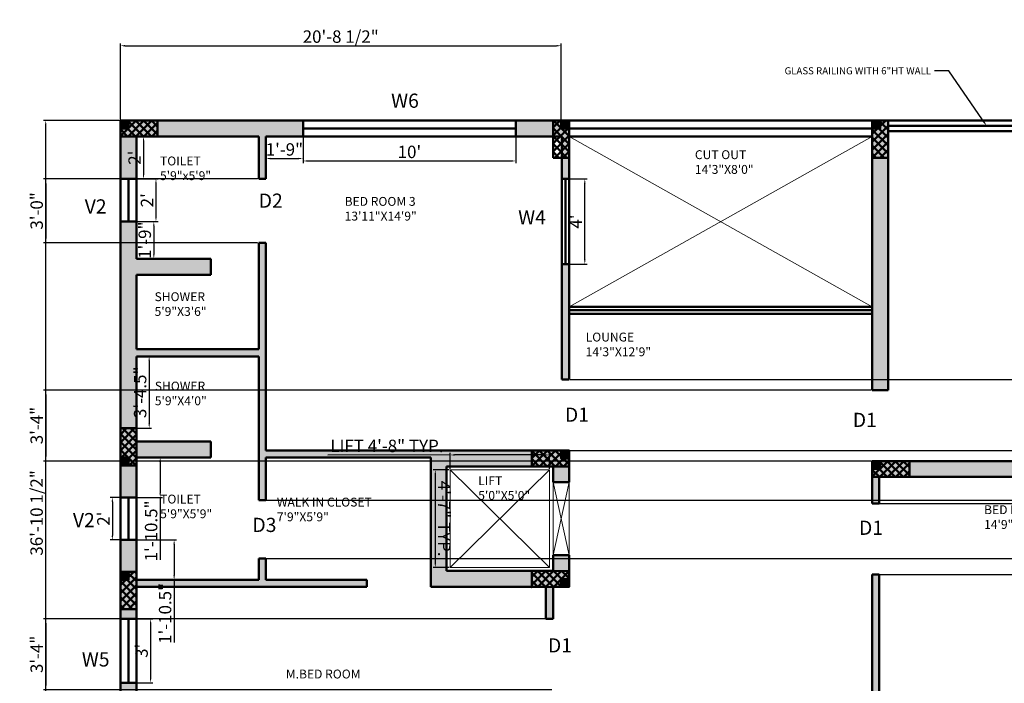
# Model space of a CAD drawing. Units: inches. Extents: x 1749 to 3550, y 1117 to 2383.
# Tile 14 of 15: x 2688 to 3244, y 1992 to 2366. Entities that reach past the tile are written whole.
import ezdxf
from ezdxf import colors
from ezdxf.entities.mleader import LeaderData, LeaderLine
from ezdxf.math import Vec2, Vec3

# ---------------------------------------------------------------- set-up
doc = ezdxf.new("R2010")
doc.units = ezdxf.units.IN
for name, color, linetype, lineweight in [('A-ANNO-DIMS', 2, 'Continuous', 18), ('A-ANNO-SYMB', 1, 'Continuous', 18), ('A-ANNO-TEXT', 3, 'Continuous', 18), ('A-AREA-IDEN', 7, 'Continuous', 18), ('A-COLS', 10, 'Continuous', 50), ('A-EQPM', 8, 'Continuous', 18), ('A-WALL', 7, 'Continuous', 50), ('A-WALL-PATT', 8, 'Continuous', 13)]:
    doc.layers.add(name, color=color, linetype=linetype, lineweight=lineweight)
doc.styles.get("Standard").update_dxf_attribs({"font": 'arial.ttf'})
doc.dimstyles.new('ISO-25', dxfattribs={"dimtxt": 7, "dimasz": 2.5, "dimexe": 1.25, "dimexo": 0.625, "dimtad": 1, "dimdec": 1, "dimlunit": 3, "dimtxsty": 'Standard', "dimcen": 2.5, "dimadec": 0, "dimazin": 0, "dimtfac": 1, "dimtdec": 1, "dimtmove": 0, "dimatfit": 3, "dimfxl": 1, "dimarcsym": 0})

# ---------------------------------------------------------------- blocks, each defined once
blk = doc.blocks.new('*D121')
at = {"layer": 'A-ANNO-DIMS', "color": 0, "lineweight": -2, "ltscale": 0.5, "transparency": 16777216}
for p, q in [((2827.22, 2300.06), (2827.22, 2286.96)), ((2848.22, 2300.06), (2848.22, 2286.96)), ((2829.72, 2288.21), (2845.72, 2288.21))]:
    blk.add_line(p, q, dxfattribs=at)
at = {"layer": 'A-ANNO-DIMS', "color": 0, "ltscale": 0.5, "transparency": 16777216}
for points in [[(2829.72, 2288.62), (2829.72, 2287.79), (2827.22, 2288.21)], [(2845.72, 2288.62), (2845.72, 2287.79), (2848.22, 2288.21)]]:
    blk.add_solid(points, dxfattribs=at)
at = {"layer": 'Defpoints', "color": 0, "ltscale": 0.5, "transparency": 16777216}
for p in [(2827.22, 2300.68), (2848.22, 2300.68), (2848.22, 2288.21)]:
    blk.add_point(p, dxfattribs=at)
at = {"layer": 'A-ANNO-DIMS', "color": 0, "ltscale": 0.5, "transparency": 16777216, "insert": (2837.72, 2292.41), "char_height": 7, "attachment_point": 5}
blk.add_mtext('1\'-9"', dxfattribs=at)
blk = doc.blocks.new('*D122')
at = {"layer": 'A-ANNO-DIMS', "color": 0, "lineweight": -2, "ltscale": 0.5, "transparency": 16777216}
for p, q in [((2848.22, 2300.06), (2848.22, 2285.58)), ((2968.22, 2300.06), (2968.22, 2285.58)), ((2850.72, 2286.83), (2965.72, 2286.83))]:
    blk.add_line(p, q, dxfattribs=at)
at = {"layer": 'A-ANNO-DIMS', "color": 0, "ltscale": 0.5, "transparency": 16777216}
for points in [[(2850.72, 2287.24), (2850.72, 2286.41), (2848.22, 2286.83)], [(2965.72, 2287.24), (2965.72, 2286.41), (2968.22, 2286.83)]]:
    blk.add_solid(points, dxfattribs=at)
at = {"layer": 'Defpoints', "color": 0, "ltscale": 0.5, "transparency": 16777216}
for p in [(2848.22, 2300.68), (2968.22, 2300.68), (2968.22, 2286.83)]:
    blk.add_point(p, dxfattribs=at)
at = {"layer": 'A-ANNO-DIMS', "color": 0, "ltscale": 0.5, "transparency": 16777216, "insert": (2908.22, 2291.03), "char_height": 7, "attachment_point": 5}
blk.add_mtext("10'", dxfattribs=at)
blk = doc.blocks.new('*D123')
at = {"layer": 'A-ANNO-DIMS', "color": 0, "lineweight": -2, "ltscale": 0.5, "transparency": 16777216}
for p, q in [((2754.84, 2300.68), (2759.52, 2300.68)), ((2758.27, 2298.18), (2758.27, 2279.18)), ((2754.84, 2276.68), (2759.52, 2276.68))]:
    blk.add_line(p, q, dxfattribs=at)
at = {"layer": 'A-ANNO-DIMS', "color": 0, "ltscale": 0.5, "transparency": 16777216}
for points in [[(2757.85, 2298.18), (2758.68, 2298.18), (2758.27, 2300.68)], [(2757.85, 2279.18), (2758.68, 2279.18), (2758.27, 2276.68)]]:
    blk.add_solid(points, dxfattribs=at)
at = {"layer": 'Defpoints', "color": 0, "ltscale": 0.5, "transparency": 16777216}
for p in [(2754.22, 2300.68), (2754.22, 2276.68), (2758.27, 2276.68)]:
    blk.add_point(p, dxfattribs=at)
at = {"layer": 'A-ANNO-DIMS', "color": 0, "ltscale": 0.5, "transparency": 16777216, "insert": (2754.13, 2288.68), "char_height": 7, "attachment_point": 5, "rotation": 90}
blk.add_mtext("2'", dxfattribs=at)
blk = doc.blocks.new('*D124')
at = {"layer": 'A-ANNO-DIMS', "color": 0, "lineweight": -2, "ltscale": 0.5, "transparency": 16777216}
for p, q in [((2754.84, 2276.68), (2766.53, 2276.68)), ((2765.28, 2274.18), (2765.28, 2255.18)), ((2754.84, 2252.68), (2766.53, 2252.68))]:
    blk.add_line(p, q, dxfattribs=at)
at = {"layer": 'A-ANNO-DIMS', "color": 0, "ltscale": 0.5, "transparency": 16777216}
for points in [[(2764.86, 2274.18), (2765.69, 2274.18), (2765.28, 2276.68)], [(2764.86, 2255.18), (2765.69, 2255.18), (2765.28, 2252.68)]]:
    blk.add_solid(points, dxfattribs=at)
at = {"layer": 'Defpoints', "color": 0, "ltscale": 0.5, "transparency": 16777216}
for p in [(2754.22, 2276.68), (2754.22, 2252.68), (2765.28, 2252.68)]:
    blk.add_point(p, dxfattribs=at)
at = {"layer": 'A-ANNO-DIMS', "color": 0, "ltscale": 0.5, "transparency": 16777216, "insert": (2761.14, 2264.68), "char_height": 7, "attachment_point": 5, "rotation": 90}
blk.add_mtext("2'", dxfattribs=at)
blk = doc.blocks.new('*D125')
at = {"layer": 'A-ANNO-DIMS', "color": 0, "lineweight": -2, "ltscale": 0.5, "transparency": 16777216}
for p, q in [((2754.84, 2252.68), (2765.33, 2252.68)), ((2764.08, 2250.18), (2764.08, 2234.18)), ((2754.84, 2231.68), (2765.33, 2231.68))]:
    blk.add_line(p, q, dxfattribs=at)
at = {"layer": 'A-ANNO-DIMS', "color": 0, "ltscale": 0.5, "transparency": 16777216}
for points in [[(2763.66, 2250.18), (2764.49, 2250.18), (2764.08, 2252.68)], [(2763.66, 2234.18), (2764.49, 2234.18), (2764.08, 2231.68)]]:
    blk.add_solid(points, dxfattribs=at)
at = {"layer": 'Defpoints', "color": 0, "ltscale": 0.5, "transparency": 16777216}
for p in [(2754.22, 2252.68), (2754.22, 2231.68), (2764.08, 2231.68)]:
    blk.add_point(p, dxfattribs=at)
at = {"layer": 'A-ANNO-DIMS', "color": 0, "ltscale": 0.5, "transparency": 16777216, "insert": (2759.88, 2242.18), "char_height": 7, "attachment_point": 5, "rotation": 90}
blk.add_mtext('1\'-9"', dxfattribs=at)
blk = doc.blocks.new('*D126')
at = {"layer": 'A-ANNO-DIMS', "color": 0, "lineweight": -2, "ltscale": 0.5, "transparency": 16777216}
for p, q in [((2754.84, 2176.68), (2762.7, 2176.68)), ((2761.45, 2174.18), (2761.45, 2138.68)), ((2754.84, 2136.18), (2762.7, 2136.18))]:
    blk.add_line(p, q, dxfattribs=at)
at = {"layer": 'A-ANNO-DIMS', "color": 0, "ltscale": 0.5, "transparency": 16777216}
for points in [[(2761.03, 2174.18), (2761.87, 2174.18), (2761.45, 2176.68)], [(2761.03, 2138.68), (2761.87, 2138.68), (2761.45, 2136.18)]]:
    blk.add_solid(points, dxfattribs=at)
at = {"layer": 'Defpoints', "color": 0, "ltscale": 0.5, "transparency": 16777216}
for p in [(2754.22, 2176.68), (2754.22, 2136.18), (2761.45, 2136.18)]:
    blk.add_point(p, dxfattribs=at)
at = {"layer": 'A-ANNO-DIMS', "color": 0, "ltscale": 0.5, "transparency": 16777216, "insert": (2757.25, 2156.43), "char_height": 7, "attachment_point": 5, "rotation": 90}
blk.add_mtext('3\'-4.5"', dxfattribs=at)
blk = doc.blocks.new('*D127')
at = {"layer": 'A-ANNO-DIMS', "color": 0, "lineweight": -2, "ltscale": 0.5, "transparency": 16777216}
for p, q in [((2754.84, 2119.68), (2768.9, 2119.68)), ((2767.65, 2117.18), (2767.65, 2099.68)), ((2754.84, 2097.18), (2768.9, 2097.18)), ((2767.65, 2097.18), (2767.65, 2061.89))]:
    blk.add_line(p, q, dxfattribs=at)
at = {"layer": 'A-ANNO-DIMS', "color": 0, "ltscale": 0.5, "transparency": 16777216}
for points in [[(2767.24, 2117.18), (2768.07, 2117.18), (2767.65, 2119.68)], [(2767.24, 2099.68), (2768.07, 2099.68), (2767.65, 2097.18)]]:
    blk.add_solid(points, dxfattribs=at)
at = {"layer": 'Defpoints', "color": 0, "ltscale": 0.5, "transparency": 16777216}
for p in [(2754.22, 2119.68), (2754.22, 2097.18), (2767.65, 2097.18)]:
    blk.add_point(p, dxfattribs=at)
at = {"layer": 'A-ANNO-DIMS', "color": 0, "ltscale": 0.5, "transparency": 16777216, "insert": (2763.45, 2078.28), "char_height": 7, "attachment_point": 5, "rotation": 90}
blk.add_mtext('1\'-10.5"', dxfattribs=at)
blk = doc.blocks.new('*D128')
at = {"layer": 'A-ANNO-DIMS', "color": 0, "lineweight": -2, "ltscale": 0.5, "transparency": 16777216}
for p, q in [((2744.59, 2097.18), (2739.43, 2097.18)), ((2740.68, 2094.68), (2740.68, 2075.68)), ((2744.59, 2073.18), (2739.43, 2073.18))]:
    blk.add_line(p, q, dxfattribs=at)
at = {"layer": 'A-ANNO-DIMS', "color": 0, "ltscale": 0.5, "transparency": 16777216}
for points in [[(2740.26, 2094.68), (2741.09, 2094.68), (2740.68, 2097.18)], [(2740.26, 2075.68), (2741.09, 2075.68), (2740.68, 2073.18)]]:
    blk.add_solid(points, dxfattribs=at)
at = {"layer": 'Defpoints', "color": 0, "ltscale": 0.5, "transparency": 16777216}
for p in [(2745.22, 2097.18), (2740.68, 2073.18), (2745.22, 2073.18)]:
    blk.add_point(p, dxfattribs=at)
at = {"layer": 'A-ANNO-DIMS', "color": 0, "ltscale": 0.5, "transparency": 16777216, "insert": (2736.54, 2085.18), "char_height": 7, "attachment_point": 5, "rotation": 90}
blk.add_mtext("2'", dxfattribs=at)
blk = doc.blocks.new('*D129')
at = {"layer": 'A-ANNO-DIMS', "color": 0, "lineweight": -2, "ltscale": 0.5, "transparency": 16777216}
for p, q in [((2754.84, 2073.18), (2776.78, 2073.18)), ((2775.53, 2070.68), (2775.53, 2053.18)), ((2754.84, 2050.68), (2776.78, 2050.68)), ((2775.53, 2050.68), (2775.53, 2015.39))]:
    blk.add_line(p, q, dxfattribs=at)
at = {"layer": 'A-ANNO-DIMS', "color": 0, "ltscale": 0.5, "transparency": 16777216}
for points in [[(2775.11, 2070.68), (2775.94, 2070.68), (2775.53, 2073.18)], [(2775.11, 2053.18), (2775.94, 2053.18), (2775.53, 2050.68)]]:
    blk.add_solid(points, dxfattribs=at)
at = {"layer": 'Defpoints', "color": 0, "ltscale": 0.5, "transparency": 16777216}
for p in [(2754.22, 2073.18), (2754.22, 2050.68), (2775.53, 2050.68)]:
    blk.add_point(p, dxfattribs=at)
at = {"layer": 'A-ANNO-DIMS', "color": 0, "ltscale": 0.5, "transparency": 16777216, "insert": (2771.33, 2031.78), "char_height": 7, "attachment_point": 5, "rotation": 90}
blk.add_mtext('1\'-10.5"', dxfattribs=at)
blk = doc.blocks.new('*D130')
at = {"layer": 'A-ANNO-DIMS', "color": 0, "lineweight": -2, "ltscale": 0.5, "transparency": 16777216}
for p, q in [((2754.84, 2028.68), (2763.51, 2028.68)), ((2762.26, 2026.18), (2762.26, 1995.18)), ((2754.84, 1992.68), (2763.51, 1992.68))]:
    blk.add_line(p, q, dxfattribs=at)
at = {"layer": 'A-ANNO-DIMS', "color": 0, "ltscale": 0.5, "transparency": 16777216}
for points in [[(2761.85, 2026.18), (2762.68, 2026.18), (2762.26, 2028.68)], [(2761.85, 1995.18), (2762.68, 1995.18), (2762.26, 1992.68)]]:
    blk.add_solid(points, dxfattribs=at)
at = {"layer": 'Defpoints', "color": 0, "ltscale": 0.5, "transparency": 16777216}
for p in [(2754.22, 2028.68), (2754.22, 1992.68), (2762.26, 1992.68)]:
    blk.add_point(p, dxfattribs=at)
at = {"layer": 'A-ANNO-DIMS', "color": 0, "ltscale": 0.5, "transparency": 16777216, "insert": (2758.06, 2010.68), "char_height": 7, "attachment_point": 5, "rotation": 90}
blk.add_mtext("3'", dxfattribs=at)
blk = doc.blocks.new('*D137')
at = {"layer": 'A-ANNO-DIMS', "color": 0, "lineweight": -2, "ltscale": 0.5, "transparency": 16777216}
for p, q in [((2998.84, 2276.68), (3008.38, 2276.68)), ((3007.13, 2231.18), (3007.13, 2274.18)), ((2998.84, 2228.68), (3008.38, 2228.68))]:
    blk.add_line(p, q, dxfattribs=at)
at = {"layer": 'A-ANNO-DIMS', "color": 0, "ltscale": 0.5, "transparency": 16777216}
for points in [[(3006.71, 2274.18), (3007.55, 2274.18), (3007.13, 2276.68)], [(3006.71, 2231.18), (3007.55, 2231.18), (3007.13, 2228.68)]]:
    blk.add_solid(points, dxfattribs=at)
at = {"layer": 'Defpoints', "color": 0, "ltscale": 0.5, "transparency": 16777216}
for p in [(2998.22, 2276.68), (3007.13, 2276.68), (2998.22, 2228.68)]:
    blk.add_point(p, dxfattribs=at)
at = {"layer": 'A-ANNO-DIMS', "color": 0, "ltscale": 0.5, "transparency": 16777216, "insert": (3003, 2252.68), "char_height": 7, "attachment_point": 5, "rotation": 90}
blk.add_mtext("4'", dxfattribs=at)
blk = doc.blocks.new('LIFT-B')
at = {"ltscale": 0.5}
for p, q in [((0, 55), (56, 55)), ((0, 0), (0, 55)), ((56, 55), (0, 0)), ((0, 55), (56, 0)), ((56, 55), (56, 0)), ((56, 0), (0, 0))]:
    blk.add_line(p, q, dxfattribs=at)
blk = doc.blocks.new('*D155')
at = {"layer": 'A-ANNO-DIMS', "color": 0, "lineweight": -2, "ltscale": 0.5, "transparency": 16777216}
for p, q in [((2931.22, 2113.31), (2931.22, 2122.33)), ((2987.22, 2113.31), (2987.22, 2122.33)), ((2931.22, 2121.08), (2862.29, 2121.07)), ((2984.72, 2121.08), (2933.72, 2121.08))]:
    blk.add_line(p, q, dxfattribs=at)
at = {"layer": 'A-ANNO-DIMS', "color": 0, "ltscale": 0.5, "transparency": 16777216}
for points in [[(2933.72, 2121.5), (2933.72, 2120.66), (2931.22, 2121.08)], [(2984.72, 2121.5), (2984.72, 2120.67), (2987.22, 2121.08)]]:
    blk.add_solid(points, dxfattribs=at)
at = {"layer": 'Defpoints', "color": 0, "ltscale": 0.5, "transparency": 16777216}
for p in [(2931.22, 2121.08), (2931.22, 2112.68), (2987.22, 2112.68)]:
    blk.add_point(p, dxfattribs=at)
at = {"layer": 'A-ANNO-DIMS', "color": 0, "ltscale": 0.5, "transparency": 16777216, "insert": (2895.51, 2125.28), "char_height": 7, "attachment_point": 5, "rotation": 0.0046}
blk.add_mtext('LIFT 4\'-8" TYP.', dxfattribs=at)
blk = doc.blocks.new('*D156')
at = {"layer": 'A-ANNO-DIMS', "color": 0, "lineweight": -2, "ltscale": 0.5, "transparency": 16777216}
for p, q in [((2930.6, 2112.68), (2921.57, 2112.68)), ((2922.82, 2110.18), (2922.83, 2060.18)), ((2930.6, 2057.68), (2921.58, 2057.68))]:
    blk.add_line(p, q, dxfattribs=at)
at = {"layer": 'A-ANNO-DIMS', "color": 0, "ltscale": 0.5, "transparency": 16777216}
for points in [[(2923.24, 2110.18), (2922.41, 2110.18), (2922.82, 2112.68)], [(2923.24, 2060.18), (2922.41, 2060.18), (2922.83, 2057.68)]]:
    blk.add_solid(points, dxfattribs=at)
at = {"layer": 'Defpoints', "color": 0, "ltscale": 0.5, "transparency": 16777216}
for p in [(2931.22, 2112.68), (2922.83, 2057.68), (2931.23, 2057.68)]:
    blk.add_point(p, dxfattribs=at)
at = {"layer": 'A-ANNO-DIMS', "color": 0, "ltscale": 0.5, "transparency": 16777216, "insert": (2926.95, 2085.18), "char_height": 7, "attachment_point": 5, "rotation": 270.0046}
blk.add_mtext('4\'-7" TYP.', dxfattribs=at)
blk = doc.blocks.new('*D181')
at = {"layer": 'A-ANNO-DIMS', "color": 0, "lineweight": -2, "ltscale": 0.5, "transparency": 16777216}
for p, q in [((2744.59, 2309.68), (2701.86, 2309.68)), ((2703.11, 1869.68), (2703.11, 2307.18)), ((2744.59, 1867.18), (2701.86, 1867.18))]:
    blk.add_line(p, q, dxfattribs=at)
at = {"layer": 'A-ANNO-DIMS', "color": 0, "ltscale": 0.5, "transparency": 16777216}
for points in [[(2702.69, 2307.18), (2703.52, 2307.18), (2703.11, 2309.68)], [(2702.69, 1869.68), (2703.52, 1869.68), (2703.11, 1867.18)]]:
    blk.add_solid(points, dxfattribs=at)
at = {"layer": 'Defpoints', "color": 0, "ltscale": 0.5, "transparency": 16777216}
for p in [(2703.11, 2309.68), (2745.22, 2309.68), (2745.22, 1867.18)]:
    blk.add_point(p, dxfattribs=at)
at = {"layer": 'A-ANNO-DIMS', "color": 0, "ltscale": 0.5, "transparency": 16777216, "insert": (2698.86, 2088.43), "char_height": 7, "attachment_point": 5, "rotation": 90}
blk.add_mtext('36\'-10 1/2"', dxfattribs=at)
blk = doc.blocks.new('*D182')
at = {"layer": 'A-ANNO-DIMS', "color": 0, "lineweight": -2, "ltscale": 0.5, "transparency": 16777216}
for p, q in [((2745.22, 2310.31), (2745.22, 2353.03)), ((2747.72, 2351.78), (2991.22, 2351.78)), ((2993.72, 2310.31), (2993.72, 2353.03))]:
    blk.add_line(p, q, dxfattribs=at)
at = {"layer": 'A-ANNO-DIMS', "color": 0, "ltscale": 0.5, "transparency": 16777216}
for points in [[(2747.72, 2352.2), (2747.72, 2351.36), (2745.22, 2351.78)], [(2991.22, 2352.2), (2991.22, 2351.36), (2993.72, 2351.78)]]:
    blk.add_solid(points, dxfattribs=at)
at = {"layer": 'Defpoints', "color": 0, "ltscale": 0.5, "transparency": 16777216}
for p in [(2993.72, 2351.78), (2745.22, 2309.68), (2993.72, 2309.68)]:
    blk.add_point(p, dxfattribs=at)
at = {"layer": 'A-ANNO-DIMS', "color": 0, "ltscale": 0.5, "transparency": 16777216, "insert": (2869.47, 2356.03), "char_height": 7, "attachment_point": 5}
blk.add_mtext('20\'-8 1/2"', dxfattribs=at)
blk = doc.blocks.new('*D191')
at = {"layer": 'A-ANNO-DIMS', "color": 0, "lineweight": -2, "ltscale": 0.5, "transparency": 16777216}
for p, q in [((2998.84, 2163.68), (3455.57, 2163.68)), ((3454.32, 2161.18), (3454.32, 2126.18)), ((2998.84, 2123.68), (3455.57, 2123.68))]:
    blk.add_line(p, q, dxfattribs=at)
at = {"layer": 'A-ANNO-DIMS', "color": 0, "ltscale": 0.5, "transparency": 16777216}
for points in [[(3453.9, 2161.18), (3454.74, 2161.18), (3454.32, 2163.68)], [(3453.9, 2126.18), (3454.74, 2126.18), (3454.32, 2123.68)]]:
    blk.add_solid(points, dxfattribs=at)
at = {"layer": 'Defpoints', "color": 0, "ltscale": 0.5, "transparency": 16777216}
for p in [(2998.22, 2163.68), (2998.22, 2123.68), (3454.32, 2123.68)]:
    blk.add_point(p, dxfattribs=at)
at = {"layer": 'A-ANNO-DIMS', "color": 0, "ltscale": 0.5, "transparency": 16777216, "insert": (3450.12, 2143.68), "char_height": 7, "attachment_point": 5, "rotation": 90}
blk.add_mtext('3\'-4"', dxfattribs=at)
blk = doc.blocks.new('*D192')
at = {"layer": 'A-ANNO-DIMS', "color": 0, "lineweight": -2, "ltscale": 0.5, "transparency": 16777216}
for p, q in [((3168.59, 2157.68), (2701.86, 2157.68)), ((2703.11, 2155.18), (2703.11, 2120.18)), ((3168.59, 2117.68), (2701.86, 2117.68))]:
    blk.add_line(p, q, dxfattribs=at)
at = {"layer": 'A-ANNO-DIMS', "color": 0, "ltscale": 0.5, "transparency": 16777216}
for points in [[(2702.69, 2155.18), (2703.52, 2155.18), (2703.11, 2157.68)], [(2702.69, 2120.18), (2703.52, 2120.18), (2703.11, 2117.68)]]:
    blk.add_solid(points, dxfattribs=at)
at = {"layer": 'Defpoints', "color": 0, "ltscale": 0.5, "transparency": 16777216}
for p in [(3169.22, 2157.68), (2703.11, 2117.68), (3169.22, 2117.68)]:
    blk.add_point(p, dxfattribs=at)
at = {"layer": 'A-ANNO-DIMS', "color": 0, "ltscale": 0.5, "transparency": 16777216, "insert": (2698.91, 2137.68), "char_height": 7, "attachment_point": 5, "rotation": 90}
blk.add_mtext('3\'-4"', dxfattribs=at)
blk = doc.blocks.new('*D193')
at = {"layer": 'A-ANNO-DIMS', "color": 0, "lineweight": -2, "ltscale": 0.5, "transparency": 16777216}
for p, q in [((3169.84, 2093.68), (3455.57, 2093.68)), ((3454.32, 2091.18), (3454.32, 2056.18)), ((3169.84, 2053.68), (3455.57, 2053.68))]:
    blk.add_line(p, q, dxfattribs=at)
at = {"layer": 'A-ANNO-DIMS', "color": 0, "ltscale": 0.5, "transparency": 16777216}
for points in [[(3453.9, 2091.18), (3454.74, 2091.18), (3454.32, 2093.68)], [(3453.9, 2056.18), (3454.74, 2056.18), (3454.32, 2053.68)]]:
    blk.add_solid(points, dxfattribs=at)
at = {"layer": 'Defpoints', "color": 0, "ltscale": 0.5, "transparency": 16777216}
for p in [(3169.22, 2093.68), (3169.22, 2053.68), (3454.32, 2053.68)]:
    blk.add_point(p, dxfattribs=at)
at = {"layer": 'A-ANNO-DIMS', "color": 0, "ltscale": 0.5, "transparency": 16777216, "insert": (3450.12, 2073.68), "char_height": 7, "attachment_point": 5, "rotation": 90}
blk.add_mtext('3\'-4"', dxfattribs=at)
blk = doc.blocks.new('*D194')
at = {"layer": 'A-ANNO-DIMS', "color": 0, "lineweight": -2, "ltscale": 0.5, "transparency": 16777216}
for p, q in [((2988.59, 2028.68), (2701.86, 2028.68)), ((2703.11, 2026.18), (2703.11, 1991.18)), ((2988.59, 1988.68), (2701.86, 1988.68))]:
    blk.add_line(p, q, dxfattribs=at)
at = {"layer": 'A-ANNO-DIMS', "color": 0, "ltscale": 0.5, "transparency": 16777216}
for points in [[(2702.69, 2026.18), (2703.52, 2026.18), (2703.11, 2028.68)], [(2702.69, 1991.18), (2703.52, 1991.18), (2703.11, 1988.68)]]:
    blk.add_solid(points, dxfattribs=at)
at = {"layer": 'Defpoints', "color": 0, "ltscale": 0.5, "transparency": 16777216}
for p in [(2989.22, 2028.68), (2703.11, 1988.68), (2989.22, 1988.68)]:
    blk.add_point(p, dxfattribs=at)
at = {"layer": 'A-ANNO-DIMS', "color": 0, "ltscale": 0.5, "transparency": 16777216, "insert": (2698.91, 2008.68), "char_height": 7, "attachment_point": 5, "rotation": 90}
blk.add_mtext('3\'-4"', dxfattribs=at)
blk = doc.blocks.new('*D195')
at = {"layer": 'A-ANNO-DIMS', "color": 0, "lineweight": -2, "ltscale": 0.5, "transparency": 16777216}
for p, q in [((2822.59, 2276.68), (2701.86, 2276.68)), ((2703.11, 2274.18), (2703.11, 2243.18)), ((2822.59, 2240.68), (2701.86, 2240.68))]:
    blk.add_line(p, q, dxfattribs=at)
at = {"layer": 'A-ANNO-DIMS', "color": 0, "ltscale": 0.5, "transparency": 16777216}
for points in [[(2702.69, 2274.18), (2703.52, 2274.18), (2703.11, 2276.68)], [(2702.69, 2243.18), (2703.52, 2243.18), (2703.11, 2240.68)]]:
    blk.add_solid(points, dxfattribs=at)
at = {"layer": 'Defpoints', "color": 0, "ltscale": 0.5, "transparency": 16777216}
for p in [(2823.22, 2276.68), (2703.11, 2240.68), (2823.22, 2240.68)]:
    blk.add_point(p, dxfattribs=at)
at = {"layer": 'A-ANNO-DIMS', "color": 0, "ltscale": 0.5, "transparency": 16777216, "insert": (2698.91, 2258.68), "char_height": 7, "attachment_point": 5, "rotation": 90}
blk.add_mtext('3\'-0"', dxfattribs=at)
blk = doc.blocks.new('*D197')
at = {"layer": 'A-ANNO-DIMS', "color": 0, "lineweight": -2, "ltscale": 0.5, "transparency": 16777216}
for p, q in [((2823.84, 2095.68), (3455.57, 2095.68)), ((3454.32, 2093.18), (3454.32, 2065.18)), ((2823.84, 2062.68), (3455.57, 2062.68))]:
    blk.add_line(p, q, dxfattribs=at)
at = {"layer": 'A-ANNO-DIMS', "color": 0, "ltscale": 0.5, "transparency": 16777216}
for points in [[(3453.9, 2093.18), (3454.74, 2093.18), (3454.32, 2095.68)], [(3453.9, 2065.18), (3454.74, 2065.18), (3454.32, 2062.68)]]:
    blk.add_solid(points, dxfattribs=at)
at = {"layer": 'Defpoints', "color": 0, "ltscale": 0.5, "transparency": 16777216}
for p in [(2823.22, 2095.68), (2823.22, 2062.68), (3454.32, 2062.68)]:
    blk.add_point(p, dxfattribs=at)
at = {"layer": 'A-ANNO-DIMS', "color": 0, "ltscale": 0.5, "transparency": 16777216, "insert": (3450.12, 2079.18), "char_height": 7, "attachment_point": 5, "rotation": 90}
blk.add_mtext('2\'-9"', dxfattribs=at)

msp = doc.modelspace()

# ---------------------------------------------------------------- hatches: boundary and pattern name
at = {"layer": 'A-COLS', "ltscale": 10}
h = msp.add_hatch(color=256, dxfattribs=at)
h.dxf.hatch_style = 1
h.paths.add_polyline_path([(2745.22, 2305.18), (2749.72, 2305.18), (2749.72, 2309.68), (2745.22, 2309.68)])
h = msp.add_hatch(dxfattribs=at)
h.set_pattern_fill('ANSI37', color=256, angle=180)
h.set_pattern_definition([(225, (4417.464, 3667.787), (2.245064, -2.245064), []), (315, (4417.464, 3667.787), (2.245064, 2.245064), [])])
h.paths.add_polyline_path([(2745.22, 2309.68), (2745.22, 2300.68), (2766.22, 2300.68), (2766.22, 2309.68)])
h = msp.add_hatch(dxfattribs=at)
h.set_pattern_fill('ANSI37', color=256, angle=90)
h.set_pattern_definition([(135, (4356.3257, 637.4367), (-2.245064, -2.245064), []), (225, (4356.3257, 637.4367), (2.245064, -2.245064), [])])
h.paths.add_polyline_path([(2998.22, 2309.68), (2989.22, 2309.68), (2989.22, 2288.68), (2998.22, 2288.68)])
h = msp.add_hatch(color=256, dxfattribs=at)
h.dxf.hatch_style = 1
h.paths.add_polyline_path([(2993.72, 2309.68), (2993.72, 2305.18), (2998.22, 2305.18), (2998.22, 2309.68)])
h = msp.add_hatch(color=256, dxfattribs=at)
h.dxf.hatch_style = 1
h.paths.add_polyline_path([(3169.22, 2309.68), (3169.22, 2305.18), (3173.72, 2305.18), (3173.72, 2309.68)])
h = msp.add_hatch(dxfattribs=at)
h.set_pattern_fill('ANSI37', color=256, angle=90)
h.set_pattern_definition([(135, (4508.4704, 637.4367), (-2.245064, -2.245064), []), (225, (4508.4704, 637.4367), (2.245064, -2.245064), [])])
h.paths.add_polyline_path([(3169.22, 2288.68), (3178.22, 2288.68), (3178.22, 2309.68), (3169.22, 2309.68)])
h = msp.add_hatch(dxfattribs=at)
h.set_pattern_fill('ANSI37', color=256, angle=270)
h.set_pattern_definition([(315, (1387.1012, 3787.4255), (2.245064, 2.245064), []), (45, (1387.1012, 3787.4255), (-2.245064, 2.245064), [])])
h.paths.add_polyline_path([(2745.21, 2115.18), (2754.21, 2115.18), (2754.21, 2136.18), (2745.21, 2136.18)])
h = msp.add_hatch(dxfattribs=at)
h.set_pattern_fill('ANSI37', color=256, angle=180)
h.set_pattern_definition([(225, (4694.5, 3481.787), (2.245064, -2.245064), []), (315, (4694.5, 3481.787), (2.245064, 2.245064), [])])
h.paths.add_polyline_path([(2977.22, 2123.68), (2977.22, 2114.68), (2998.22, 2114.68), (2998.22, 2123.68)])
h = msp.add_hatch(color=256, dxfattribs=at)
h.dxf.hatch_style = 1
h.paths.add_polyline_path([(2998.22, 2123.68), (2993.72, 2123.68), (2993.72, 2119.18), (2998.22, 2119.18)])
h = msp.add_hatch(color=256, dxfattribs=at)
h.dxf.hatch_style = 1
h.paths.add_polyline_path([(2749.71, 2115.18), (2749.71, 2119.68), (2745.21, 2119.68), (2745.21, 2115.18)])
h = msp.add_hatch(color=256, dxfattribs=at)
h.dxf.hatch_style = 1
h.paths.add_polyline_path([(3169.22, 2113.18), (3173.72, 2113.18), (3173.72, 2117.68), (3169.22, 2117.68)])
h = msp.add_hatch(dxfattribs=at)
h.set_pattern_fill('ANSI37', color=256, angle=180)
h.set_pattern_definition([(225, (4841.464, 3475.787), (2.245064, -2.245064), []), (315, (4841.464, 3475.787), (2.245064, 2.245064), [])])
h.paths.add_polyline_path([(3169.22, 2117.68), (3169.22, 2108.68), (3190.22, 2108.68), (3190.22, 2117.68)])
h = msp.add_hatch(color=256, dxfattribs=at)
h.dxf.hatch_style = 1
h.paths.add_polyline_path([(2745.22, 2055.15), (2745.22, 2050.65), (2749.72, 2050.65), (2749.72, 2055.15)])
h = msp.add_hatch(dxfattribs=at)
h.set_pattern_fill('ANSI37', color=256, angle=90)
h.set_pattern_definition([(135, (4079.926, 382.902), (-2.245064, -2.245064), []), (225, (4079.926, 382.902), (2.245064, -2.245064), [])])
h.paths.add_polyline_path([(2745.22, 2034.15), (2754.22, 2034.15), (2754.22, 2055.15), (2745.22, 2055.15)])
h = msp.add_hatch(dxfattribs=at)
h.set_pattern_fill('ANSI37', color=256, angle=0.3283)
h.set_pattern_definition([(45.32827, (1333.7838, 679.0164), (-2.25789, 2.2321643), []), (135.32827, (1333.7838, 679.0164), (-2.2321643, -2.25789), [])])
h.paths.add_polyline_path([(2998.22, 2046.68), (2998.17, 2055.68), (2977.17, 2055.56), (2977.22, 2046.56)])
h = msp.add_hatch(color=256, dxfattribs=at)
h.dxf.hatch_style = 1
h.paths.add_polyline_path([(2998.19, 2051.18), (2993.69, 2051.16), (2993.72, 2046.66), (2998.22, 2046.68)])
at = {"layer": 'A-WALL-PATT', "ltscale": 0.5}
h = msp.add_hatch(color=256, dxfattribs=at)
h.dxf.hatch_style = 1
h.paths.add_polyline_path([(2745.22, 2309.68), (2745.22, 2276.68), (2754.22, 2276.68), (2754.22, 2300.68), (2823.22, 2300.68), (2823.22, 2276.68), (2827.22, 2276.68), (2827.22, 2300.68), (2848.22, 2300.68), (2848.22, 2309.68)])
h = msp.add_hatch(color=256, dxfattribs=at)
h.dxf.hatch_style = 1
h.paths.add_polyline_path([(2968.22, 2309.68), (2968.22, 2300.68), (2994.22, 2300.68), (2994.22, 2276.68), (2998.22, 2276.68), (2998.22, 2300.68), (2998.22, 2309.68)])
h = msp.add_hatch(color=256, dxfattribs=at)
h.dxf.hatch_style = 1
h.paths.add_polyline_path([(3169.22, 2157.68), (3178.22, 2157.68), (3178.22, 2303.68), (3178.22, 2309.68), (3169.22, 2309.68), (3169.22, 2300.68), (3169.22, 2204.68), (3169.22, 2200.68)])
h = msp.add_hatch(color=256, dxfattribs=at)
h.dxf.hatch_style = 1
h.paths.add_polyline_path([(2929.22, 2055.68), (2929.22, 2114.68), (2989.22, 2114.68), (2989.22, 2105.68), (2998.22, 2105.68), (2998.22, 2123.68), (2827.22, 2123.68), (2827.22, 2240.68), (2823.22, 2240.68), (2823.22, 2231.68), (2823.22, 2222.68), (2823.22, 2180.68), (2754.22, 2180.68), (2754.22, 2222.68), (2796.22, 2222.68), (2796.22, 2231.68), (2754.22, 2231.68), (2754.22, 2252.68), (2745.22, 2252.68), (2745.22, 2097.18), (2754.22, 2097.18), (2754.22, 2119.68), (2796.22, 2119.68), (2796.22, 2128.68), (2754.22, 2128.68), (2754.22, 2176.68), (2823.22, 2176.68), (2823.22, 2128.68), (2823.22, 2119.68), (2823.22, 2095.68), (2827.22, 2095.68), (2827.22, 2119.68), (2920.22, 2119.68), (2920.22, 2046.68), (2985.22, 2046.68), (2985.22, 2028.68), (2989.22, 2028.68), (2989.22, 2046.68), (2998.22, 2046.68), (2998.22, 2064.68), (2989.22, 2064.68), (2989.22, 2055.68)])
h = msp.add_hatch(color=256, dxfattribs=at)
h.dxf.hatch_style = 1
h.paths.add_polyline_path([(2994.22, 2163.68), (2998.22, 2163.68), (2998.22, 2200.68), (2998.22, 2204.68), (2998.22, 2228.68), (2994.22, 2228.68)])
h = msp.add_hatch(color=256, dxfattribs=at)
h.dxf.hatch_style = 1
h.paths.add_polyline_path([(3289.22, 2108.68), (3350.22, 2108.68), (3350.22, 2093.68), (3359.22, 2093.68), (3359.22, 2108.68), (3412.22, 2108.68), (3412.22, 2117.68), (3289.22, 2117.68), (3178.22, 2117.68), (3169.22, 2117.68), (3169.22, 2093.68), (3173.22, 2093.68), (3173.22, 2108.68)])
h = msp.add_hatch(color=256, dxfattribs=at)
h.dxf.hatch_style = 1
h.paths.add_polyline_path([(2754.22, 2073.18), (2745.22, 2073.18), (2745.22, 2028.68), (2754.22, 2028.68), (2754.22, 2046.68), (2884.22, 2046.68), (2884.22, 2050.68), (2827.22, 2050.68), (2827.22, 2062.68), (2823.22, 2062.68), (2823.22, 2050.68), (2754.22, 2050.68)])
h = msp.add_hatch(color=256, dxfattribs=at)
h.dxf.hatch_style = 1
h.paths.add_polyline_path([(3303.22, 1968.68), (3289.22, 1968.68), (3173.22, 1968.68), (3173.22, 2053.68), (3169.22, 2053.68), (3169.22, 1964.68), (3169.22, 1890.68), (3163.22, 1890.68), (3163.22, 1881.68), (3169.22, 1881.68), (3169.22, 1867.18), (3243.72, 1867.18), (3243.72, 1876.18), (3173.22, 1876.18), (3173.22, 1964.68), (3289.22, 1964.68), (3293.22, 1964.68), (3293.22, 1958.68), (3297.22, 1958.68), (3297.22, 1964.68), (3303.22, 1964.68)])
h = msp.add_hatch(color=256, dxfattribs=at)
h.dxf.hatch_style = 1
h.paths.add_polyline_path([(2754.22, 1876.18), (2754.22, 1992.68), (2745.22, 1992.68), (2745.22, 1881.68), (2745.22, 1867.18), (2902.72, 1867.18), (2902.72, 1876.18)])

# ---------------------------------------------------------------- linework, layer by layer
at = {"layer": 'A-ANNO-SYMB', "ltscale": 0.5}
for p, q in [((2998.22, 2300.68), (3169.22, 2204.68)), ((3169.22, 2300.68), (2998.22, 2204.68))]:
    msp.add_line(p, q, dxfattribs=at)
at = {"layer": 'A-COLS', "ltscale": 10}
for points in [[(2745.22, 2305.18), (2745.22, 2309.68), (2749.72, 2309.68), (2749.72, 2305.18)], [(2766.22, 2300.68), (2745.22, 2300.68), (2745.22, 2309.68), (2766.22, 2309.68)], [(2989.22, 2288.68), (2989.22, 2309.68), (2998.22, 2309.68), (2998.22, 2288.68)], [(2993.72, 2309.68), (2998.22, 2309.68), (2998.22, 2305.18), (2993.72, 2305.18)], [(3173.72, 2309.68), (3169.22, 2309.68), (3169.22, 2305.18), (3173.72, 2305.18)], [(3178.22, 2288.68), (3178.22, 2309.68), (3169.22, 2309.68), (3169.22, 2288.68)], [(2754.21, 2136.18), (2754.21, 2115.18), (2745.21, 2115.18), (2745.21, 2136.18)], [(2977.22, 2114.68), (2998.22, 2114.68), (2998.22, 2123.68), (2977.22, 2123.68)], [(2998.22, 2119.18), (2998.22, 2123.68), (2993.72, 2123.68), (2993.72, 2119.18)], [(2749.71, 2115.18), (2745.21, 2115.18), (2745.21, 2119.68), (2749.71, 2119.68)], [(3169.22, 2113.18), (3169.22, 2117.68), (3173.72, 2117.68), (3173.72, 2113.18)], [(3190.22, 2108.68), (3169.22, 2108.68), (3169.22, 2117.68), (3190.22, 2117.68)], [(2749.72, 2055.15), (2745.22, 2055.15), (2745.22, 2050.65), (2749.72, 2050.65)], [(2754.22, 2034.15), (2754.22, 2055.15), (2745.22, 2055.15), (2745.22, 2034.15)], [(2977.17, 2055.56), (2998.17, 2055.68), (2998.22, 2046.68), (2977.22, 2046.56)], [(2998.19, 2051.18), (2998.22, 2046.68), (2993.72, 2046.66), (2993.69, 2051.16)]]:
    msp.add_lwpolyline(points, close=True, dxfattribs=at)
at = {"layer": 'A-EQPM', "ltscale": 0.5}
for p, q in [((2998.22, 2105.68), (2989.22, 2105.68)), ((2989.22, 2105.68), (2989.22, 2064.68)), ((2998.22, 2064.68), (2989.22, 2105.68)), ((2989.22, 2105.68), (2998.22, 2105.68)), ((2998.22, 2105.68), (2989.22, 2064.68)), ((2998.22, 2064.68), (2998.22, 2105.68)), ((2989.22, 2064.68), (2998.22, 2064.68))]:
    msp.add_line(p, q, dxfattribs=at)
at = {"layer": 'A-WALL', "ltscale": 0.5}
for p, q in [((2745.22, 2309.68), (3412.22, 2309.68)), ((2745.22, 2309.68), (2745.22, 1881.68)), ((2848.22, 2300.68), (2848.22, 2309.68)), ((2848.22, 2305.18), (2968.22, 2305.18)), ((2968.22, 2300.68), (2968.22, 2309.68)), ((2998.22, 2300.68), (2998.22, 2309.68)), ((2998.22, 2305.18), (3169.22, 2305.18)), ((3169.22, 2300.68), (3169.22, 2309.68)), ((3178.22, 2303.68), (3178.22, 2309.68)), ((3178.22, 2306.68), (3289.22, 2306.68)), ((2754.22, 2300.68), (2823.22, 2300.68)), ((2754.22, 2300.68), (2754.22, 2231.68)), ((2823.22, 2300.68), (2823.22, 2276.68)), ((2827.22, 2300.68), (2827.22, 2276.68)), ((2827.22, 2300.68), (2994.22, 2300.68)), ((2994.22, 2300.68), (2994.22, 2163.68)), ((2998.22, 2300.68), (2998.22, 2204.68)), ((2998.22, 2300.68), (3169.22, 2300.68)), ((3169.22, 2300.68), (3169.22, 2204.68)), ((3178.22, 2303.68), (3178.22, 2157.68)), ((3178.22, 2303.68), (3289.22, 2303.68)), ((2754.22, 2276.68), (2745.22, 2276.68)), ((2749.72, 2276.68), (2749.72, 2252.68)), ((2823.22, 2276.68), (2827.22, 2276.68)), ((2998.22, 2276.68), (2994.22, 2276.68)), ((2996.22, 2276.68), (2996.22, 2228.68)), ((2754.22, 2252.68), (2745.22, 2252.68)), ((2823.22, 2240.68), (2827.22, 2240.68)), ((2823.22, 2240.68), (2823.22, 2231.68)), ((2827.22, 2240.68), (2827.22, 2123.68)), ((2754.22, 2231.68), (2796.22, 2231.68)), ((2796.22, 2222.68), (2796.22, 2231.68)), ((2823.22, 2222.68), (2823.22, 2231.68)), ((2998.22, 2228.68), (2994.22, 2228.68)), ((2754.22, 2222.68), (2796.22, 2222.68)), ((2754.22, 2222.68), (2754.22, 2180.68)), ((2823.22, 2222.68), (2823.22, 2180.68)), ((2998.22, 2204.68), (3169.22, 2204.68)), ((2998.22, 2204.68), (2998.22, 2200.68)), ((3169.22, 2204.68), (3169.22, 2200.68)), ((2998.22, 2202.68), (3169.22, 2202.68)), ((2998.22, 2200.68), (3169.22, 2200.68)), ((2998.22, 2200.68), (2998.22, 2163.68)), ((3169.22, 2200.68), (3169.22, 2157.68)), ((2754.22, 2180.68), (2823.22, 2180.68)), ((2754.22, 2176.68), (2823.22, 2176.68)), ((2754.22, 2176.68), (2754.22, 2128.68)), ((2823.22, 2176.68), (2823.22, 2128.68)), ((2994.22, 2163.68), (2998.22, 2163.68)), ((3178.22, 2157.68), (3169.22, 2157.68)), ((2754.22, 2128.68), (2796.22, 2128.68)), ((2796.22, 2119.68), (2796.22, 2128.68)), ((2823.22, 2119.68), (2823.22, 2128.68)), ((2827.22, 2123.68), (2998.22, 2123.68)), ((2998.22, 2123.68), (2998.22, 2105.68)), ((2754.22, 2119.68), (2796.22, 2119.68)), ((2754.22, 2119.68), (2754.22, 2050.68)), ((2823.22, 2119.68), (2823.22, 2095.68)), ((2827.22, 2119.68), (2920.22, 2119.68)), ((2827.22, 2119.68), (2827.22, 2095.68)), ((2920.22, 2119.68), (2920.22, 2046.68)), ((3178.22, 2117.68), (3169.22, 2117.68)), ((3169.22, 2117.68), (3169.22, 2093.68)), ((3178.22, 2117.68), (3289.22, 2117.68)), ((2929.22, 2114.68), (2929.22, 2055.68)), ((2929.22, 2114.68), (2989.22, 2114.68)), ((2989.22, 2114.68), (2989.22, 2105.68)), ((2989.22, 2105.68), (2998.22, 2105.68)), ((3173.22, 2108.68), (3289.22, 2108.68)), ((3173.22, 2108.68), (3173.22, 2093.68)), ((2754.22, 2097.18), (2745.22, 2097.18)), ((2749.72, 2097.18), (2749.72, 2073.18)), ((2823.22, 2095.68), (2827.22, 2095.68)), ((3173.22, 2093.68), (3169.22, 2093.68)), ((2754.22, 2073.18), (2745.22, 2073.18)), ((2823.22, 2062.68), (2827.22, 2062.68)), ((2823.22, 2062.68), (2823.22, 2050.68)), ((2827.22, 2062.68), (2827.22, 2050.68)), ((2989.22, 2064.68), (2998.22, 2064.68)), ((2989.22, 2064.68), (2989.22, 2055.68)), ((2998.22, 2064.68), (2998.22, 2046.68)), ((2989.22, 2055.68), (2929.22, 2055.68)), ((2754.22, 2050.68), (2823.22, 2050.68)), ((2827.22, 2050.68), (2884.22, 2050.68)), ((2884.22, 2046.68), (2884.22, 2050.68)), ((3173.22, 2053.68), (3169.22, 2053.68)), ((3169.22, 2053.68), (3169.22, 1964.68)), ((3173.22, 2053.68), (3173.22, 1968.68)), ((2754.22, 2046.68), (2884.22, 2046.68)), ((2754.22, 2046.68), (2754.22, 1876.18)), ((2985.22, 2046.68), (2920.22, 2046.68)), ((2925.22, 2046.68), (2985.22, 2046.68)), ((2985.22, 2046.68), (2985.22, 2028.68)), ((2989.22, 2046.68), (2989.22, 2028.68)), ((2998.22, 2046.68), (2989.22, 2046.68)), ((2754.22, 2028.68), (2745.22, 2028.68)), ((2749.72, 2028.68), (2749.72, 1992.68)), ((2985.22, 2028.68), (2989.22, 2028.68)), ((2754.22, 1992.68), (2745.22, 1992.68))]:
    msp.add_line(p, q, dxfattribs=at)

# ---------------------------------------------------------------- block references
at = {"layer": 'A-EQPM', "rotation": 180.0046290675699}
msp.add_blockref('LIFT-B', (2987.22, 2112.68), dxfattribs=at)

# ---------------------------------------------------------------- texts
at = {"layer": 'A-ANNO-TEXT', "ltscale": 0.5}
for s, p in [('W6', (2897.89, 2316.79)), ('D2', (2823.22, 2260.45)), ('V2', (2725.1, 2257.21)), ('W4', (2969.54, 2251.08)), ('D1', (2995.9, 2139.79)), ('D1', (3158.26, 2136.86)), ('V2', (2718.44, 2080.35)), ('D3', (2819.66, 2077.66)), ('D1', (3161.78, 2076.05)), ('D1', (2986.34, 2009.75)), ('W5', (2723.46, 2001.84))]:
    msp.add_text(s, height=8, dxfattribs=at).set_placement(p)
at = {"layer": 'A-AREA-IDEN', "ltscale": 0.5}
for s, p in [('TOILET', (2767.55, 2284.33)), ('CUT OUT', (3069.22, 2287.87)), ('14\'3"X8\'0"', (3069.22, 2279.57)), ('5\'9"x5\'9"', (2767.55, 2276.03)), ('BED ROOM 3', (2871.68, 2261.54)), ('13\'11"X14\'9"', (2871.68, 2253.24)), ('SHOWER', (2764.49, 2207.8)), ('5\'9"X3\'6"', (2764.49, 2199.5)), ('LOUNGE', (3007.62, 2185.05)), ('14\'3"X12\'9"', (3007.62, 2176.75)), ('SHOWER', (2764.62, 2157.42)), ('5\'9"X4\'0"', (2764.62, 2149.12)), ('LIFT', (2947.03, 2104.08)), ('5\'0"X5\'0"', (2947.03, 2095.78)), ('TOILET', (2767.65, 2093.73)), ('WALK IN CLOSET', (2833.46, 2092.01)), ('5\'9"X5\'9"', (2767.65, 2085.43)), ('7\'9"X5\'9"', (2833.46, 2083.71)), ('BED ROOM 4', (3232.33, 2087.73)), ('14\'9"X11\'8"', (3232.33, 2079.43)), ('M.BED ROOM', (2838.52, 1995.1))]:
    msp.add_text(s, height=5, dxfattribs=at).set_placement(p)

# ---------------------------------------------------------------- dimensions: what is measured, and where the dimension line sits
at = {"layer": 'A-ANNO-DIMS', "ltscale": 0.5}
for base, p1, p2, override, picture, middle in [((2993.72, 2351.78), (2745.22, 2309.68), (2993.72, 2309.68), {"dimdec": 1, "dimlfac": 1, "dimrnd": 0, "dimzin": 1, "dimdsep": 46, "dimlunit": 4, "dimfrac": 2}, '*D182', (2869.47, 2356.03)), ((2848.22, 2288.21), (2827.22, 2300.68), (2848.22, 2300.68), {"dimclrd": 0, "dimclre": 0, "dimclrt": 0}, '*D121', (2837.72, 2292.41)), ((2968.22, 2286.83), (2848.22, 2300.68), (2968.22, 2300.68), {"dimclrd": 0, "dimclre": 0, "dimclrt": 0}, '*D122', (2908.22, 2291.03))]:
    dim = msp.add_linear_dim(base=base, p1=p1, p2=p2, dimstyle='ISO-25', override=override, dxfattribs=at)
    dim.commit()
    dim.dimension.update_dxf_attribs({"geometry": picture, "text_midpoint": middle})
for base, p1, p2, override, picture, middle in [((2703.11, 2309.68), (2745.22, 1867.18), (2745.22, 2309.68), {"dimdec": 1, "dimlfac": 1, "dimrnd": 0, "dimzin": 1, "dimdsep": 46, "dimlunit": 4, "dimfrac": 2}, '*D181', (2698.86, 2088.43)), ((2758.27, 2276.68), (2754.22, 2300.68), (2754.22, 2276.68), {"dimclrd": 0, "dimclre": 0, "dimclrt": 0}, '*D123', (2754.13, 2288.68)), ((2703.11, 2240.68), (2823.22, 2276.68), (2823.22, 2240.68), {"dimdec": 1, "dimlfac": 1, "dimrnd": 0, "dimzin": 1, "dimdsep": 46, "dimlunit": 4, "dimfrac": 2}, '*D195', (2698.91, 2258.68)), ((2765.28, 2252.68), (2754.22, 2276.68), (2754.22, 2252.68), {"dimclrd": 0, "dimclre": 0, "dimclrt": 0}, '*D124', (2761.14, 2264.68)), ((3007.13, 2276.68), (2998.22, 2228.68), (2998.22, 2276.68), {"dimclrd": 0, "dimclre": 0, "dimclrt": 0}, '*D137', (3003, 2252.68)), ((2764.08, 2231.68), (2754.22, 2252.68), (2754.22, 2231.68), {"dimclrd": 0, "dimclre": 0, "dimclrt": 0}, '*D125', (2759.88, 2242.18)), ((2761.45, 2136.18), (2754.22, 2176.68), (2754.22, 2136.18), {"dimclrd": 0, "dimclre": 0, "dimclrt": 0}, '*D126', (2757.25, 2156.43)), ((3454.32, 2123.68), (2998.22, 2163.68), (2998.22, 2123.68), {"dimdec": 1, "dimlfac": 1, "dimrnd": 0, "dimzin": 1, "dimdsep": 46, "dimlunit": 4, "dimfrac": 2}, '*D191', (3450.12, 2143.68)), ((2703.11, 2117.68), (3169.22, 2157.68), (3169.22, 2117.68), {"dimdec": 1, "dimlfac": 1, "dimrnd": 0, "dimzin": 1, "dimdsep": 46, "dimlunit": 4, "dimfrac": 2}, '*D192', (2698.91, 2137.68)), ((2767.65, 2097.18), (2754.22, 2119.68), (2754.22, 2097.18), {"dimclrd": 0, "dimclre": 0, "dimclrt": 0}, '*D127', (2763.45, 2078.28)), ((2740.68, 2073.18), (2745.22, 2097.18), (2745.22, 2073.18), {"dimclrd": 0, "dimclre": 0, "dimclrt": 0}, '*D128', (2736.54, 2085.18)), ((3454.32, 2062.68), (2823.22, 2095.68), (2823.22, 2062.68), {"dimdec": 1, "dimlfac": 1, "dimrnd": 0, "dimzin": 1, "dimdsep": 46, "dimlunit": 4, "dimfrac": 2}, '*D197', (3450.12, 2079.18)), ((3454.32, 2053.68), (3169.22, 2093.68), (3169.22, 2053.68), {"dimdec": 1, "dimlfac": 1, "dimrnd": 0, "dimzin": 1, "dimdsep": 46, "dimlunit": 4, "dimfrac": 2}, '*D193', (3450.12, 2073.68)), ((2775.53, 2050.68), (2754.22, 2073.18), (2754.22, 2050.68), {"dimclrd": 0, "dimclre": 0, "dimclrt": 0}, '*D129', (2771.33, 2031.78)), ((2703.11, 1988.68), (2989.22, 2028.68), (2989.22, 1988.68), {"dimdec": 1, "dimlfac": 1, "dimrnd": 0, "dimzin": 1, "dimdsep": 46, "dimlunit": 4, "dimfrac": 2}, '*D194', (2698.91, 2008.68)), ((2762.26, 1992.68), (2754.22, 2028.68), (2754.22, 1992.68), {"dimclrd": 0, "dimclre": 0, "dimclrt": 0}, '*D130', (2758.06, 2010.68))]:
    dim = msp.add_linear_dim(base=base, p1=p1, p2=p2, angle=90, dimstyle='ISO-25', override=override, dxfattribs=at)
    dim.commit()
    dim.dimension.update_dxf_attribs({"geometry": picture, "text_midpoint": middle})
for base, p1, p2, angle, text, picture, middle in [((2931.22, 2121.08), (2987.22, 2112.68), (2931.22, 2112.68), 180.0046, 'LIFT <> TYP.', '*D155', (2895.51, 2125.28)), ((2922.83, 2057.68), (2931.22, 2112.68), (2931.23, 2057.68), 270.0046, '<> TYP.', '*D156', (2926.95, 2085.18))]:
    dim = msp.add_linear_dim(base=base, p1=p1, p2=p2, angle=angle, text=text, dimstyle='ISO-25', override={"dimdec": 1, "dimrnd": 0, "dimzin": 1, "dimlunit": 4, "dimfrac": 2}, dxfattribs=at)
    dim.commit()
    dim.dimension.update_dxf_attribs({"geometry": picture, "text_midpoint": middle})

# ---------------------------------------------------------------- leaders
at = {"layer": 'A-ANNO-TEXT', "ltscale": 0.5}
ml = msp.add_multileader_mtext('Standard', dxfattribs=at)
ml.set_content('GLASS RAILING WITH 6"HT WALL', color=256)
ml.set_leader_properties()
ml.build(insert=Vec2(0, 0))
ctx = ml.context
ctx.base_point, ctx.plane_origin = Vec3(3111.66, 2337.62), Vec3(3233.72, 2306.68)
ctx.text_align_type = 2
notes = []
notes.append((ctx, [(0, (1, 1, 0), (3212.4, 2337.62), (-1, 0), 8, [(0, [(3233.72, 2306.68)], 0, [])])]))
ctx.mtext.insert, ctx.mtext.alignment, ctx.mtext.flow_direction = Vec3(3202.4, 2339.66), 3, 5
for ctx, leaders in notes:
    for number, flags, end, landing, length, lines in leaders:
        leader = LeaderData()
        leader.index, (leader.has_last_leader_line, leader.has_dogleg_vector, leader.attachment_direction) = number, flags
        leader.last_leader_point, leader.dogleg_vector, leader.dogleg_length = Vec3(end), Vec3(landing), length
        for number, points, colour, breaks in lines:
            line = LeaderLine()
            line.index, line.vertices, line.color, line.breaks = number, Vec3.list(points), colors.encode_raw_color(colour), breaks
            leader.lines.append(line)
        ctx.leaders.append(leader)

doc.saveas('drawing.dxf')
